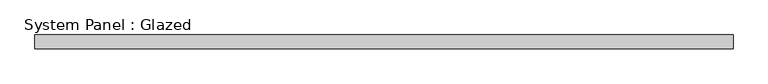
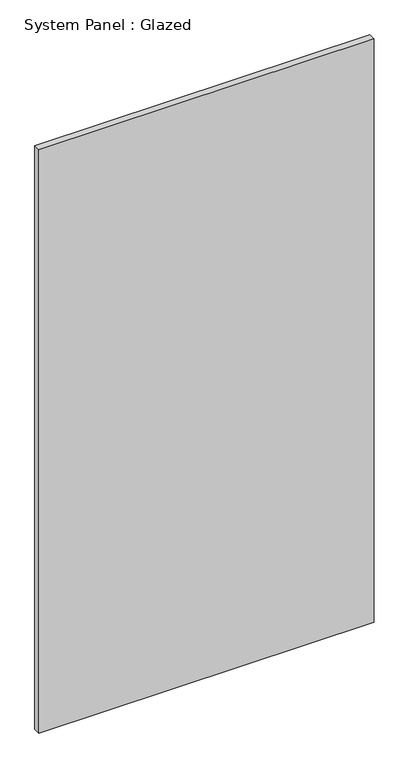
"""IFC4 building model written with IfcOpenShell, lengths in millimetres: plate geometry, System Panel : Glazed."""

from ifc_helpers import new_model, si_unit, origin, origin_with_axes, place, context, project, spatial, polyline, outline, extrude, source, transform, mapped, element, save


def system_panel_glazed_de34110e(model_context):
    return source(origin(), model_context, "Body", "SweptSolid", [
        extrude(outline(polyline([(637.0528322, 19.05), (-637.0528322, 19.05), (-637.0528322, 44.45), (637.0528322, 44.45), (637.0528322, 19.05)])), origin_with_axes(), (0.0, 0.0, 1.0), 2343.15),
    ])


if __name__ == "__main__":
    model = new_model("IFC4")
    model_context = context("Model", 3, world=origin())
    ifc_project = project(units=[si_unit("LENGTHUNIT", "METRE", prefix="MILLI")], contexts=[model_context])
    site = spatial("IfcSite", under=ifc_project)
    building = spatial("IfcBuilding", under=site)
    placement = place(None, origin())
    system_panel_glazed_shape = system_panel_glazed_de34110e(model_context)
    element("IfcPlate", 1, ObjectType="System Panel : Glazed", at=placement, inside=building, context=model_context, shape_type="MappedRepresentation", body=[
        mapped(system_panel_glazed_shape, transform((0.0, 0.0, 0.0), x_axis=(1.0, 0.0, 0.0), y_axis=(0.0, 1.0, 0.0), z_axis=(0.0, 0.0, 1.0))),
    ])
    save(model, "model.ifc")

# Revit data of these elements
# Type "System Panel : Glazed"
#   Construction Type Id = "GSP4R"
#   Analytic Construction = "1/8 in Pilkington single glazing"
#   Visual Light Transmittance = 0.9
#   Solar Heat Gain Coefficient = 0.86
#   Heat Transfer Coefficient (U) = 1.18115 BTU/(h·ft²·°F)
#   Define Thermal Properties by = 1
# Element 1 (IfcPlate, "System Panel : Glazed")
#   Materials on its faces: "Glass"
# Materials
#   "Glass": class "Glass", colour RGB 0 128 192, transparency 0.75, Description = "Soda Lime Glass", Cost = 0
